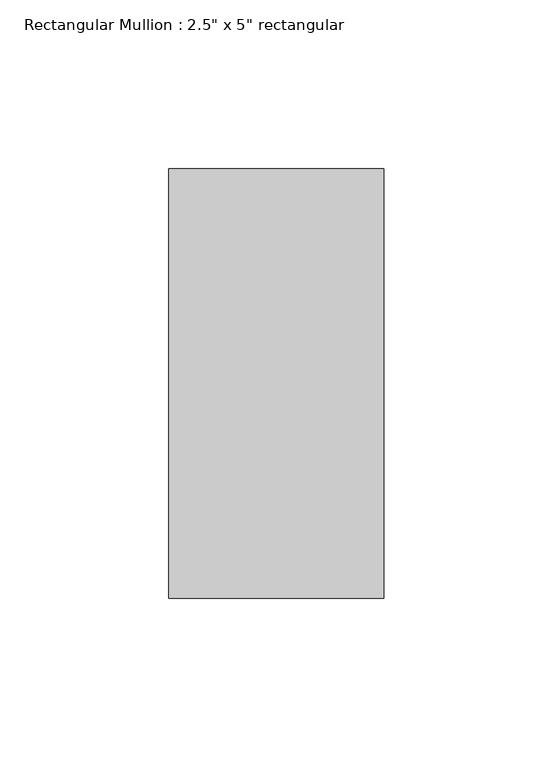
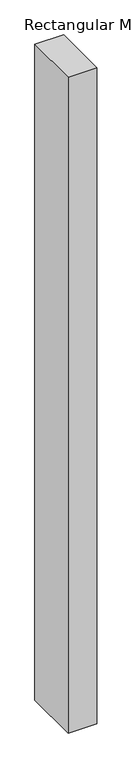
"""IFC4 building model written with IfcOpenShell, lengths in millimetres: member geometry."""

from ifc_helpers import new_model, si_unit, frame, origin, place, context, project, spatial, polyline, outline, extrude, source, transform, mapped, element, save


def member_2bcda102(model_context):
    return source(origin(), model_context, "Body", "SweptSolid", [
        extrude(outline(polyline([(0.0, 63.5), (0.0, -63.5), (-63.5, -63.5), (-63.5, 63.5), (0.0, 63.5)])), frame((0.0, 0.0, -1533.247479), z_axis=(0.0, 0.0, 1.0), x_axis=(1.0, 0.0, 0.0)), (0.0, 0.0, 1.0), 1533.247479),
    ])


if __name__ == "__main__":
    model = new_model("IFC4")
    model_context = context("Model", 3, world=origin())
    ifc_project = project(units=[si_unit("LENGTHUNIT", "METRE", prefix="MILLI")], contexts=[model_context])
    site = spatial("IfcSite", under=ifc_project)
    building = spatial("IfcBuilding", under=site)
    placement = place(None, origin())
    member_shape = member_2bcda102(model_context)
    element("IfcMember", 1, ObjectType="Rectangular Mullion : 2.5\" x 5\" rectangular", at=placement, inside=building, context=model_context, shape_type="MappedRepresentation", body=[
        mapped(member_shape, transform((0.0, 0.0, 0.0), x_axis=(1.0, 0.0, 0.0), y_axis=(0.0, 1.0, 0.0), z_axis=(0.0, 0.0, 1.0))),
    ])
    save(model, "model.ifc")

# Revit data of these elements
# Type "Rectangular Mullion : 2.5\" x 5\" rectangular"
#   built-in parameter 1007304 = 0.416667 (stored number, unit not read)
#   built-in parameter 1007301 = 0.104167 (stored number, unit not read)
#   built-in parameter 1007300 = 0.104167 (stored number, unit not read)
# Element 1 (IfcMember, "Rectangular Mullion : 2.5\" x 5\" rectangular")
#   Materials on its faces: "Aluminum"
# Materials
#   "Aluminum": class "Metal", colour RGB 247 247 247, transparency 0, Description = "Aluminum 6061", Cost = 0
